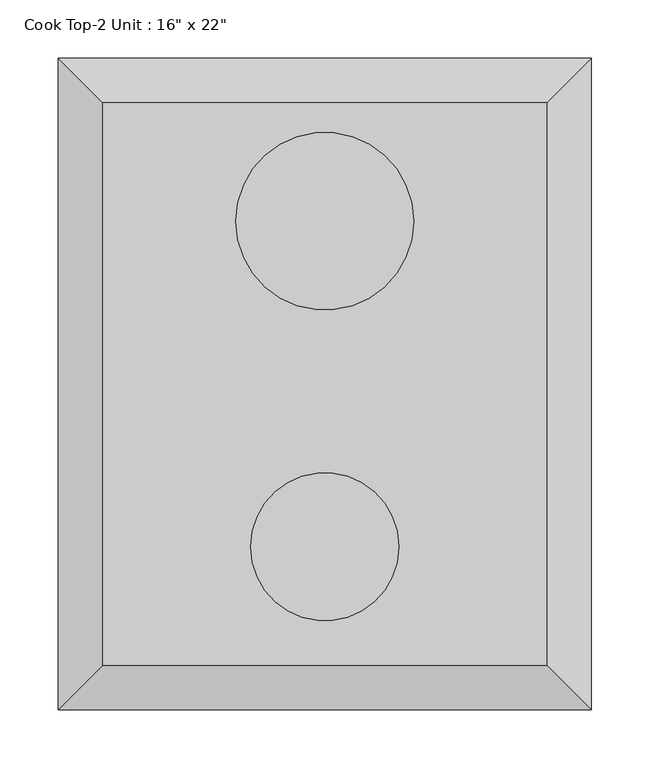
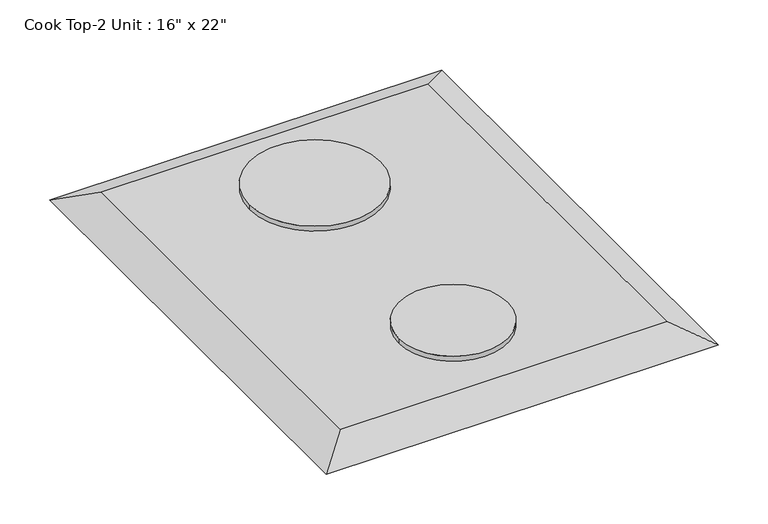
"""IFC4 building model written with IfcOpenShell, lengths in millimetres: proxy geometry."""

from ifc_helpers import new_model, si_unit, point, frame, frame_2d, origin, place, context, project, spatial, circle_curve, trimmed, segment, composite_curve, outline, extrude, faceted_brep, source, transform, mapped, element, save


def proxy_84368fe0(model_context):
    return source(origin(), model_context, "Body", "SolidModel", [
        faceted_brep([(266.7, 271.5247956, 933.45), (-114.3, 271.5247956, 933.45), (-114.3, -211.0752044, 933.45), (266.7, -211.0752044, 933.45), (304.8, 309.6247956, 914.4), (304.8, -249.1752044, 914.4), (-152.4, -249.1752044, 914.4), (-152.4, 309.6247956, 914.4)], [[[0, 1, 2, 3]], [[4, 5, 6, 7]], [[4, 7, 1, 0]], [[7, 6, 2, 1]], [[6, 5, 3, 2]], [[5, 4, 0, 3]]]),
        extrude(outline(composite_curve([segment(trimmed(circle_curve(frame_2d((76.2, 169.9247956)), 76.2), [point((152.4, 169.9247956))], [point((0.0, 169.9247956))], False, "CARTESIAN"), True, "CONTINUOUS"), segment(trimmed(circle_curve(frame_2d((76.2, 169.9247956)), 76.2), [point((0.0, 169.9247956))], [point((152.4, 169.9247956))], False, "CARTESIAN"), True, "CONTINUOUS")], self_intersect=False)), frame((0.0, 0.0, 933.45), z_axis=(0.0, 0.0, 1.0), x_axis=(1.0, 0.0, 0.0)), (0.0, 0.0, 1.0), 6.35),
        extrude(outline(composite_curve([segment(trimmed(circle_curve(frame_2d((76.2, -109.4752044)), 63.5), [point((139.7, -109.4752044))], [point((12.7, -109.4752044))], False, "CARTESIAN"), True, "CONTINUOUS"), segment(trimmed(circle_curve(frame_2d((76.2, -109.4752044)), 63.5), [point((12.7, -109.4752044))], [point((139.7, -109.4752044))], False, "CARTESIAN"), True, "CONTINUOUS")], self_intersect=False)), frame((0.0, 0.0, 933.45), z_axis=(0.0, 0.0, 1.0), x_axis=(1.0, 0.0, 0.0)), (0.0, 0.0, 1.0), 6.35),
    ])


if __name__ == "__main__":
    model = new_model("IFC4")
    model_context = context("Model", 3, world=origin())
    ifc_project = project(units=[si_unit("LENGTHUNIT", "METRE", prefix="MILLI")], contexts=[model_context])
    site = spatial("IfcSite", under=ifc_project)
    building = spatial("IfcBuilding", under=site)
    placement = place(None, origin())
    proxy_shape = proxy_84368fe0(model_context)
    element("IfcBuildingElementProxy", 1, Name="Cook Top-2 Unit : 16\" x 22\"", ObjectType="Cook Top-2 Unit : 16\" x 22\"", at=placement, inside=building, context=model_context, shape_type="MappedRepresentation", body=[
        mapped(proxy_shape, transform((0.0, 0.0, 0.0), x_axis=(1.0, 0.0, 0.0), y_axis=(0.0, 1.0, 0.0), z_axis=(0.0, 0.0, 1.0))),
    ])
    save(model, "model.ifc")

# Revit data of these elements
# Type "Cook Top-2 Unit : 16\" x 22\""
#   Assembly Code = "E1090400"
#   Counter Height = 3' - 0"
#   Depth = 1' - 10"
#   Width = 1' - 6"
#   Burner Material = Metal - Chrome
#   Cooktop Material = Metal - Steel, Polished
#   Default Elevation = 0
# Element 1 (IfcBuildingElementProxy, "Cook Top-2 Unit : 16\" x 22\"")
#   Materials on its faces: "Metal - Steel, Polished", "Metal - Chrome"
# Materials
#   "Metal - Chrome": colour RGB 57 57 57, transparency 0
#   "Metal - Steel, Polished": colour RGB 57 57 57, transparency 0
